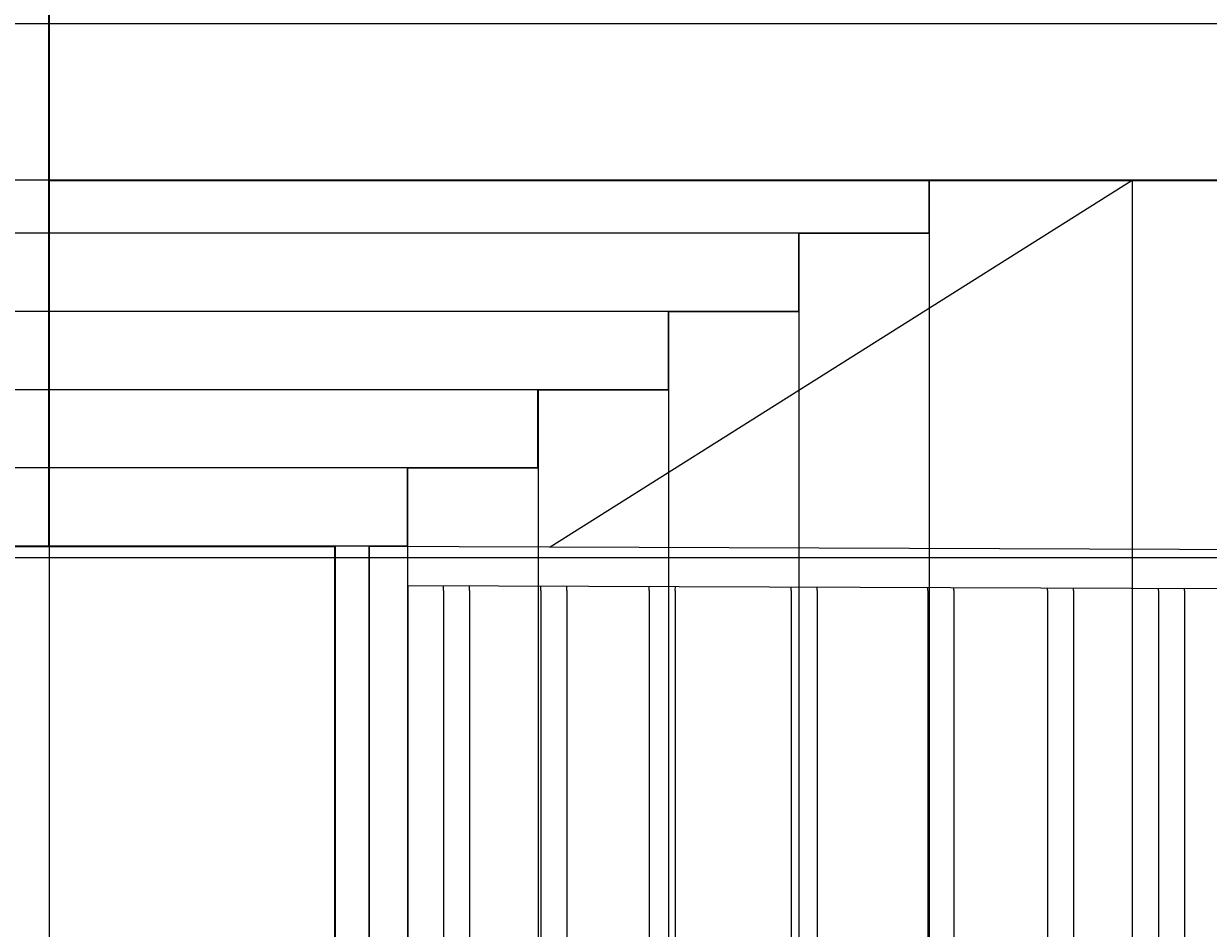
# Model space of a CAD drawing. Units: inches. Extents: x -13 to 809, y 112 to 656.
# Tile 19 of 55: x 339 to 430, y 181 to 251. Entities that reach past the tile are written whole.
import ezdxf

# ---------------------------------------------------------------- set-up
doc = ezdxf.new("R2010")
doc.units = ezdxf.units.IN
doc.header["$MEASUREMENT"] = 0
for name, color, linetype, lineweight in [('A-ANNO-DIMS', 2, 'Continuous', 18), ('A-DOOR', 4, 'Continuous', 25), ('A-ELEV', 7, 'Continuous', 35), ('A-FLOR-STRS', 3, 'Continuous', 25)]:
    doc.layers.add(name, color=color, linetype=linetype, lineweight=lineweight)
doc.styles.get("Standard").update_dxf_attribs({"font": 'arial.ttf'})
doc.dimstyles.get("Standard").update_dxf_attribs({"dimtxt": 0.625, "dimasz": 0.18, "dimexe": 0.18, "dimexo": 0.0625, "dimgap": 0.09, "dimtad": 0, "dimtih": 1, "dimtoh": 1, "dimdec": 4, "dimzin": 0, "dimdsep": 46, "dimlunit": 4, "dimtxsty": 'Standard', "dimcen": 0.09, "dimadec": 0, "dimazin": 0, "dimtfac": 1, "dimtdec": 4, "dimtofl": 0, "dimtmove": 0, "dimatfit": 3, "dimfxl": 1, "dimtolj": 1, "dimtzin": 0, "dimarcsym": 0})

# ---------------------------------------------------------------- blocks, each defined once
blk = doc.blocks.new('*D19')
at = {"layer": 'A-ANNO-DIMS', "color": 0, "lineweight": -2, "transparency": 16777216}
for p, q in [((337.507, 306.457), (337.507, 112.34)), ((365.938, 210.722), (365.938, 112.34)), ((337.687, 112.52), (350.573, 112.52)), ((365.758, 112.52), (352.873, 112.52))]:
    blk.add_line(p, q, dxfattribs=at)
at = {"layer": 'A-ANNO-DIMS', "color": 0, "transparency": 16777216}
for points in [[(337.687, 112.55), (337.687, 112.49), (337.507, 112.52)], [(365.758, 112.55), (365.758, 112.49), (365.938, 112.52)]]:
    blk.add_solid(points, dxfattribs=at)
at = {"layer": 'Defpoints', "color": 0, "transparency": 16777216}
for p in [(337.507, 306.52), (365.938, 210.785), (365.938, 112.52)]:
    blk.add_point(p, dxfattribs=at)
at = {"layer": 'A-ANNO-DIMS', "color": 0, "transparency": 16777216, "insert": (351.723, 112.52), "char_height": 0.625, "attachment_point": 5}
blk.add_mtext('\\A1;28.43', dxfattribs=at)
blk = doc.blocks.new('*D20')
at = {"layer": 'A-ANNO-DIMS', "color": 0, "lineweight": -2, "transparency": 16777216}
for p, q in [((365.938, 210.722), (365.938, 112.34)), ((607.574, 209.813), (607.574, 112.34)), ((366.118, 112.52), (485.365, 112.52)), ((607.394, 112.52), (488.148, 112.52))]:
    blk.add_line(p, q, dxfattribs=at)
at = {"layer": 'A-ANNO-DIMS', "color": 0, "transparency": 16777216}
for points in [[(366.118, 112.55), (366.118, 112.49), (365.938, 112.52)], [(607.394, 112.55), (607.394, 112.49), (607.574, 112.52)]]:
    blk.add_solid(points, dxfattribs=at)
at = {"layer": 'Defpoints', "color": 0, "transparency": 16777216}
for p in [(365.938, 210.785), (607.574, 209.875), (607.574, 112.52)]:
    blk.add_point(p, dxfattribs=at)
at = {"layer": 'A-ANNO-DIMS', "color": 0, "transparency": 16777216, "insert": (486.756, 112.52), "char_height": 0.625, "attachment_point": 5}
blk.add_mtext('\\A1;241.64', dxfattribs=at)
blk = doc.blocks.new('*D49')
at = {"layer": 'A-ANNO-DIMS', "color": 0, "lineweight": -2, "transparency": 16777216}
for p, q in [((590.946, 250.843), (-12.099, 250.843)), ((-11.919, 250.663), (-11.919, 245.247)), ((-11.919, 239.023), (-11.919, 244.439)), ((590.946, 238.843), (-12.099, 238.843))]:
    blk.add_line(p, q, dxfattribs=at)
at = {"layer": 'A-ANNO-DIMS', "color": 0, "transparency": 16777216}
for points in [[(-11.949, 250.663), (-11.889, 250.663), (-11.919, 250.843)], [(-11.949, 239.023), (-11.889, 239.023), (-11.919, 238.843)]]:
    blk.add_solid(points, dxfattribs=at)
at = {"layer": 'Defpoints', "color": 0, "transparency": 16777216}
for p in [(-11.919, 250.843), (591.008, 250.843), (591.008, 238.843)]:
    blk.add_point(p, dxfattribs=at)
at = {"layer": 'A-ANNO-DIMS', "color": 0, "transparency": 16777216, "insert": (-11.919, 244.843), "char_height": 0.625, "attachment_point": 5}
blk.add_mtext('\\A1;12', dxfattribs=at)
blk = doc.blocks.new('*D50')
at = {"layer": 'A-ANNO-DIMS', "color": 0, "lineweight": -2, "transparency": 16777216}
for p, q in [((590.946, 238.843), (-12.099, 238.843)), ((-11.919, 238.663), (-11.919, 224.768)), ((-11.919, 210.055), (-11.919, 223.95)), ((607.512, 209.875), (-12.099, 209.875))]:
    blk.add_line(p, q, dxfattribs=at)
at = {"layer": 'A-ANNO-DIMS', "color": 0, "transparency": 16777216}
for points in [[(-11.949, 238.663), (-11.889, 238.663), (-11.919, 238.843)], [(-11.949, 210.055), (-11.889, 210.055), (-11.919, 209.875)]]:
    blk.add_solid(points, dxfattribs=at)
at = {"layer": 'Defpoints', "color": 0, "transparency": 16777216}
for p in [(591.008, 238.843), (-11.919, 209.875), (607.574, 209.875)]:
    blk.add_point(p, dxfattribs=at)
at = {"layer": 'A-ANNO-DIMS', "color": 0, "transparency": 16777216, "insert": (-11.919, 224.359), "char_height": 0.625, "attachment_point": 5}
blk.add_mtext('\\A1;28.97', dxfattribs=at)
blk = doc.blocks.new('*D51')
at = {"layer": 'A-ANNO-DIMS', "color": 0, "lineweight": -2, "transparency": 16777216}
for p, q in [((341.407, 288.388), (341.407, 112.34)), ((442.184, 288.388), (442.184, 112.34)), ((341.587, 112.52), (390.437, 112.52)), ((442.004, 112.52), (393.154, 112.52))]:
    blk.add_line(p, q, dxfattribs=at)
at = {"layer": 'A-ANNO-DIMS', "color": 0, "transparency": 16777216}
for points in [[(341.587, 112.55), (341.587, 112.49), (341.407, 112.52)], [(442.004, 112.55), (442.004, 112.49), (442.184, 112.52)]]:
    blk.add_solid(points, dxfattribs=at)
at = {"layer": 'Defpoints', "color": 0, "transparency": 16777216}
for p in [(341.407, 288.451), (442.184, 288.451), (442.184, 112.52)]:
    blk.add_point(p, dxfattribs=at)
at = {"layer": 'A-ANNO-DIMS', "color": 0, "transparency": 16777216, "insert": (391.796, 112.52), "char_height": 0.625, "attachment_point": 5}
blk.add_mtext('\\A1;100.78', dxfattribs=at)
blk = doc.blocks.new('*D74')
at = {"layer": 'A-ANNO-DIMS', "color": 0, "lineweight": -2, "transparency": 16777216}
for p, q in [((341.407, 210.722), (341.407, 112.34)), ((368.897, 210.711), (368.897, 112.34)), ((341.587, 112.52), (354.001, 112.52)), ((368.717, 112.52), (356.302, 112.52))]:
    blk.add_line(p, q, dxfattribs=at)
at = {"layer": 'A-ANNO-DIMS', "color": 0, "transparency": 16777216}
for points in [[(341.587, 112.55), (341.587, 112.49), (341.407, 112.52)], [(368.717, 112.55), (368.717, 112.49), (368.897, 112.52)]]:
    blk.add_solid(points, dxfattribs=at)
at = {"layer": 'Defpoints', "color": 0, "transparency": 16777216}
for p in [(341.407, 210.785), (368.897, 210.774), (368.897, 112.52)]:
    blk.add_point(p, dxfattribs=at)
at = {"layer": 'A-ANNO-DIMS', "color": 0, "transparency": 16777216, "insert": (355.152, 112.52), "char_height": 0.625, "attachment_point": 5}
blk.add_mtext('\\A1;27.49', dxfattribs=at)
blk = doc.blocks.new('*D75')
at = {"layer": 'A-ANNO-DIMS', "color": 0, "lineweight": -2, "transparency": 16777216}
for p, q in [((378.897, 222.711), (378.897, 112.34)), ((368.897, 216.711), (368.897, 112.34)), ((369.077, 112.52), (373.389, 112.52)), ((378.717, 112.52), (374.404, 112.52))]:
    blk.add_line(p, q, dxfattribs=at)
at = {"layer": 'A-ANNO-DIMS', "color": 0, "transparency": 16777216}
for points in [[(369.077, 112.55), (369.077, 112.49), (368.897, 112.52)], [(378.717, 112.55), (378.717, 112.49), (378.897, 112.52)]]:
    blk.add_solid(points, dxfattribs=at)
at = {"layer": 'Defpoints', "color": 0, "transparency": 16777216}
for p in [(378.897, 222.774), (368.897, 216.774), (378.897, 112.52)]:
    blk.add_point(p, dxfattribs=at)
at = {"layer": 'A-ANNO-DIMS', "color": 0, "transparency": 16777216, "insert": (373.897, 112.52), "char_height": 0.625, "attachment_point": 5}
blk.add_mtext('\\A1;10', dxfattribs=at)
blk = doc.blocks.new('*D76')
at = {"layer": 'A-ANNO-DIMS', "color": 0, "lineweight": -2, "transparency": 16777216}
for p, q in [((388.897, 228.711), (388.897, 112.34)), ((378.897, 222.711), (378.897, 112.34)), ((379.077, 112.52), (383.389, 112.52)), ((388.717, 112.52), (384.404, 112.52))]:
    blk.add_line(p, q, dxfattribs=at)
at = {"layer": 'A-ANNO-DIMS', "color": 0, "transparency": 16777216}
for points in [[(379.077, 112.55), (379.077, 112.49), (378.897, 112.52)], [(388.717, 112.55), (388.717, 112.49), (388.897, 112.52)]]:
    blk.add_solid(points, dxfattribs=at)
at = {"layer": 'Defpoints', "color": 0, "transparency": 16777216}
for p in [(388.897, 228.774), (378.897, 222.774), (388.897, 112.52)]:
    blk.add_point(p, dxfattribs=at)
at = {"layer": 'A-ANNO-DIMS', "color": 0, "transparency": 16777216, "insert": (383.897, 112.52), "char_height": 0.625, "attachment_point": 5}
blk.add_mtext('\\A1;10', dxfattribs=at)
blk = doc.blocks.new('*D77')
at = {"layer": 'A-ANNO-DIMS', "color": 0, "lineweight": -2, "transparency": 16777216}
for p, q in [((398.897, 234.711), (398.897, 112.34)), ((388.897, 228.711), (388.897, 112.34)), ((389.077, 112.52), (393.389, 112.52)), ((398.717, 112.52), (394.404, 112.52))]:
    blk.add_line(p, q, dxfattribs=at)
at = {"layer": 'A-ANNO-DIMS', "color": 0, "transparency": 16777216}
for points in [[(389.077, 112.55), (389.077, 112.49), (388.897, 112.52)], [(398.717, 112.55), (398.717, 112.49), (398.897, 112.52)]]:
    blk.add_solid(points, dxfattribs=at)
at = {"layer": 'Defpoints', "color": 0, "transparency": 16777216}
for p in [(398.897, 234.774), (388.897, 228.774), (398.897, 112.52)]:
    blk.add_point(p, dxfattribs=at)
at = {"layer": 'A-ANNO-DIMS', "color": 0, "transparency": 16777216, "insert": (393.897, 112.52), "char_height": 0.625, "attachment_point": 5}
blk.add_mtext('\\A1;10', dxfattribs=at)
blk = doc.blocks.new('*D78')
at = {"layer": 'A-ANNO-DIMS', "color": 0, "lineweight": -2, "transparency": 16777216}
for p, q in [((408.897, 238.78), (408.897, 112.34)), ((398.897, 234.711), (398.897, 112.34)), ((399.077, 112.52), (403.389, 112.52)), ((408.717, 112.52), (404.404, 112.52))]:
    blk.add_line(p, q, dxfattribs=at)
at = {"layer": 'A-ANNO-DIMS', "color": 0, "transparency": 16777216}
for points in [[(399.077, 112.55), (399.077, 112.49), (398.897, 112.52)], [(408.717, 112.55), (408.717, 112.49), (408.897, 112.52)]]:
    blk.add_solid(points, dxfattribs=at)
at = {"layer": 'Defpoints', "color": 0, "transparency": 16777216}
for p in [(408.897, 238.843), (398.897, 234.774), (408.897, 112.52)]:
    blk.add_point(p, dxfattribs=at)
at = {"layer": 'A-ANNO-DIMS', "color": 0, "transparency": 16777216, "insert": (403.897, 112.52), "char_height": 0.625, "attachment_point": 5}
blk.add_mtext('\\A1;10', dxfattribs=at)
blk = doc.blocks.new('*D79')
at = {"layer": 'A-ANNO-DIMS', "color": 0, "lineweight": -2, "transparency": 16777216}
for p, q in [((408.897, 238.78), (408.897, 112.34)), ((424.469, 238.78), (424.469, 112.34)), ((409.077, 112.52), (415.328, 112.52)), ((424.289, 112.52), (418.037, 112.52))]:
    blk.add_line(p, q, dxfattribs=at)
at = {"layer": 'A-ANNO-DIMS', "color": 0, "transparency": 16777216}
for points in [[(409.077, 112.55), (409.077, 112.49), (408.897, 112.52)], [(424.289, 112.55), (424.289, 112.49), (424.469, 112.52)]]:
    blk.add_solid(points, dxfattribs=at)
at = {"layer": 'Defpoints', "color": 0, "transparency": 16777216}
for p in [(408.897, 238.843), (424.469, 238.843), (424.469, 112.52)]:
    blk.add_point(p, dxfattribs=at)
at = {"layer": 'A-ANNO-DIMS', "color": 0, "transparency": 16777216, "insert": (416.683, 112.52), "char_height": 0.625, "attachment_point": 5}
blk.add_mtext('\\A1;15.572', dxfattribs=at)
blk = doc.blocks.new('*D80')
at = {"layer": 'A-ANNO-DIMS', "color": 0, "lineweight": -2, "transparency": 16777216}
for p, q in [((368.834, 216.774), (-12.099, 216.774)), ((-11.919, 216.594), (-11.919, 214.183)), ((-11.919, 210.954), (-11.919, 213.365)), ((368.834, 210.774), (-12.099, 210.774))]:
    blk.add_line(p, q, dxfattribs=at)
at = {"layer": 'A-ANNO-DIMS', "color": 0, "transparency": 16777216}
for points in [[(-11.949, 216.594), (-11.889, 216.594), (-11.919, 216.774)], [(-11.949, 210.954), (-11.889, 210.954), (-11.919, 210.774)]]:
    blk.add_solid(points, dxfattribs=at)
at = {"layer": 'Defpoints', "color": 0, "transparency": 16777216}
for p in [(-11.919, 216.774), (368.897, 216.774), (368.897, 210.774)]:
    blk.add_point(p, dxfattribs=at)
at = {"layer": 'A-ANNO-DIMS', "color": 0, "transparency": 16777216, "insert": (-11.919, 213.774), "char_height": 0.625, "attachment_point": 5}
blk.add_mtext('\\A1;6', dxfattribs=at)
blk = doc.blocks.new('*D81')
at = {"layer": 'A-ANNO-DIMS', "color": 0, "lineweight": -2, "transparency": 16777216}
for p, q in [((378.834, 222.774), (-12.099, 222.774)), ((-11.919, 222.594), (-11.919, 220.183)), ((-11.919, 216.954), (-11.919, 219.365)), ((378.834, 216.774), (-12.099, 216.774))]:
    blk.add_line(p, q, dxfattribs=at)
at = {"layer": 'A-ANNO-DIMS', "color": 0, "transparency": 16777216}
for points in [[(-11.949, 222.594), (-11.889, 222.594), (-11.919, 222.774)], [(-11.949, 216.954), (-11.889, 216.954), (-11.919, 216.774)]]:
    blk.add_solid(points, dxfattribs=at)
at = {"layer": 'Defpoints', "color": 0, "transparency": 16777216}
for p in [(-11.919, 222.774), (378.897, 222.774), (378.897, 216.774)]:
    blk.add_point(p, dxfattribs=at)
at = {"layer": 'A-ANNO-DIMS', "color": 0, "transparency": 16777216, "insert": (-11.919, 219.774), "char_height": 0.625, "attachment_point": 5}
blk.add_mtext('\\A1;6', dxfattribs=at)
blk = doc.blocks.new('*D82')
at = {"layer": 'A-ANNO-DIMS', "color": 0, "lineweight": -2, "transparency": 16777216}
for p, q in [((388.834, 228.774), (-12.099, 228.774)), ((-11.919, 228.594), (-11.919, 226.183)), ((-11.919, 222.954), (-11.919, 225.365)), ((388.834, 222.774), (-12.099, 222.774))]:
    blk.add_line(p, q, dxfattribs=at)
at = {"layer": 'A-ANNO-DIMS', "color": 0, "transparency": 16777216}
for points in [[(-11.949, 228.594), (-11.889, 228.594), (-11.919, 228.774)], [(-11.949, 222.954), (-11.889, 222.954), (-11.919, 222.774)]]:
    blk.add_solid(points, dxfattribs=at)
at = {"layer": 'Defpoints', "color": 0, "transparency": 16777216}
for p in [(-11.919, 228.774), (388.897, 228.774), (388.897, 222.774)]:
    blk.add_point(p, dxfattribs=at)
at = {"layer": 'A-ANNO-DIMS', "color": 0, "transparency": 16777216, "insert": (-11.919, 225.774), "char_height": 0.625, "attachment_point": 5}
blk.add_mtext('\\A1;6', dxfattribs=at)
blk = doc.blocks.new('*D83')
at = {"layer": 'A-ANNO-DIMS', "color": 0, "lineweight": -2, "transparency": 16777216}
for p, q in [((398.834, 234.774), (-12.099, 234.774)), ((-11.919, 234.594), (-11.919, 232.183)), ((-11.919, 228.954), (-11.919, 231.365)), ((398.834, 228.774), (-12.099, 228.774))]:
    blk.add_line(p, q, dxfattribs=at)
at = {"layer": 'A-ANNO-DIMS', "color": 0, "transparency": 16777216}
for points in [[(-11.949, 234.594), (-11.889, 234.594), (-11.919, 234.774)], [(-11.949, 228.954), (-11.889, 228.954), (-11.919, 228.774)]]:
    blk.add_solid(points, dxfattribs=at)
at = {"layer": 'Defpoints', "color": 0, "transparency": 16777216}
for p in [(-11.919, 234.774), (398.897, 234.774), (398.897, 228.774)]:
    blk.add_point(p, dxfattribs=at)
at = {"layer": 'A-ANNO-DIMS', "color": 0, "transparency": 16777216, "insert": (-11.919, 231.774), "char_height": 0.625, "attachment_point": 5}
blk.add_mtext('\\A1;6', dxfattribs=at)
blk = doc.blocks.new('*D84')
at = {"layer": 'A-ANNO-DIMS', "color": 0, "lineweight": -2, "transparency": 16777216}
for p, q in [((408.834, 238.843), (-12.099, 238.843)), ((-11.919, 238.663), (-11.919, 237.217)), ((-11.919, 234.954), (-11.919, 236.399)), ((408.834, 234.774), (-12.099, 234.774))]:
    blk.add_line(p, q, dxfattribs=at)
at = {"layer": 'A-ANNO-DIMS', "color": 0, "transparency": 16777216}
for points in [[(-11.949, 238.663), (-11.889, 238.663), (-11.919, 238.843)], [(-11.949, 234.954), (-11.889, 234.954), (-11.919, 234.774)]]:
    blk.add_solid(points, dxfattribs=at)
at = {"layer": 'Defpoints', "color": 0, "transparency": 16777216}
for p in [(-11.919, 238.843), (408.897, 238.843), (408.897, 234.774)]:
    blk.add_point(p, dxfattribs=at)
at = {"layer": 'A-ANNO-DIMS', "color": 0, "transparency": 16777216, "insert": (-11.919, 236.808), "char_height": 0.625, "attachment_point": 5}
blk.add_mtext('\\A1;4.069', dxfattribs=at)

msp = doc.modelspace()

# ---------------------------------------------------------------- linework, layer by layer
at = {"layer": 'A-DOOR'}
for p, q in [((371.6498, 207.3724), (371.6513, 207.7634)), ((371.6498, 207.3724), (371.6498, 155.2141)), ((373.6498, 207.3724), (373.6513, 207.7559)), ((373.6498, 207.3724), (373.6498, 155.2141)), ((379.1123, 207.3724), (379.1136, 207.7353)), ((379.1123, 207.3724), (379.1123, 155.2141)), ((381.1123, 207.3724), (381.1136, 207.7278)), ((381.1123, 207.3724), (381.1123, 155.2141)), ((387.4276, 207.3724), (387.4288, 207.704)), ((387.4276, 207.3724), (387.4276, 155.2141)), ((389.4276, 207.3724), (389.4288, 207.6965)), ((389.4276, 207.3724), (389.4276, 155.2141)), ((398.3015, 207.3724), (398.3026, 207.6631)), ((398.3015, 207.3724), (398.3015, 155.2141)), ((400.3015, 207.3724), (400.3025, 207.6556)), ((400.3015, 207.3724), (400.3015, 155.2141)), ((408.7873, 207.3724), (408.7882, 207.6236)), ((408.7873, 207.3724), (408.7873, 155.2141)), ((410.7873, 207.3724), (410.7882, 207.6161)), ((410.7873, 207.3724), (410.7873, 155.2141)), ((417.9555, 207.3724), (417.9563, 207.5891)), ((417.9555, 207.3724), (417.9555, 155.2141)), ((419.9555, 207.3724), (419.9563, 207.5816)), ((419.9555, 207.3724), (419.9555, 155.2141)), ((426.484, 207.3724), (426.4847, 207.557)), ((426.484, 207.3724), (426.484, 155.2141)), ((428.484, 207.3724), (428.4847, 207.5495)), ((428.484, 207.3724), (428.484, 155.2141))]:
    msp.add_line(p, q, dxfattribs=at)
for points in [[(365.9383, 210.7849), (607.5741, 209.8753), (607.5741, 152.2141), (365.9383, 152.2141)], [(368.9383, 207.7736), (604.5741, 206.8866), (604.5741, 155.2141), (368.9383, 155.2141)]]:
    msp.add_lwpolyline(points, close=True, dxfattribs=at)
at = {"layer": 'A-ELEV'}
for p, q in [((341.4072, 210.7849), (341.4072, 524.281)), ((341.4072, 238.8429), (591.008, 238.8429)), ((311.6991, 210.7849), (363.3158, 210.7849)), ((363.3158, 210.7849), (363.3158, 150.5199))]:
    msp.add_line(p, q, dxfattribs=at)
at = {"layer": 'A-FLOR-STRS'}
for p, q in [((379.8204, 210.7327), (424.469, 238.8429)), ((408.8966, 234.7738), (408.8966, 238.8429)), ((398.8966, 228.7738), (398.8966, 234.7738)), ((398.8966, 234.7738), (408.8966, 234.7738)), ((388.8966, 222.7738), (388.8966, 228.7738)), ((388.8966, 228.7738), (398.8966, 228.7738)), ((378.8966, 216.7738), (378.8966, 222.7738)), ((378.8966, 222.7738), (388.8966, 222.7738)), ((368.8966, 210.7738), (368.8966, 216.7738)), ((368.8966, 216.7738), (378.8966, 216.7738))]:
    msp.add_line(p, q, dxfattribs=at)

# ---------------------------------------------------------------- dimensions: what is measured, and where the dimension line sits
at = {"layer": 'A-ANNO-DIMS'}
for base, p1, p2, override, picture, middle in [((365.9383, 112.5199), (337.5074, 306.5199), (365.9383, 210.7849), {"dimdec": 2, "dimlfac": 1, "dimrnd": 0, "dimzin": 0, "dimdsep": 46, "dimlunit": 2}, '*D19', (351.7228, 112.5199)), ((442.1845, 112.5199), (341.4072, 288.4508), (442.1845, 288.4508), {"dimdec": 2, "dimlfac": 1, "dimrnd": 0, "dimzin": 0, "dimdsep": 46, "dimlunit": 2}, '*D51', (391.7958, 112.5199)), ((408.8966, 112.5199), (398.8966, 234.7738), (408.8966, 238.8429), {"dimdec": 0, "dimlfac": 1, "dimrnd": 0, "dimzin": 0, "dimdsep": 46, "dimlunit": 2}, '*D78', (403.8966, 112.5199)), ((424.469, 112.5199), (408.8966, 238.8429), (424.469, 238.8429), {"dimdec": 3, "dimlfac": 1, "dimrnd": 0, "dimzin": 0, "dimdsep": 46, "dimlunit": 2}, '*D79', (416.6828, 112.5199)), ((398.8966, 112.5199), (388.8966, 228.7738), (398.8966, 234.7738), {"dimdec": 0, "dimlfac": 1, "dimrnd": 0, "dimzin": 0, "dimdsep": 46, "dimlunit": 2}, '*D77', (393.8966, 112.5199)), ((388.8966, 112.5199), (378.8966, 222.7738), (388.8966, 228.7738), {"dimdec": 0, "dimlfac": 1, "dimrnd": 0, "dimzin": 0, "dimdsep": 46, "dimlunit": 2}, '*D76', (383.8966, 112.5199)), ((378.8966, 112.5199), (368.8966, 216.7738), (378.8966, 222.7738), {"dimdec": 0, "dimlfac": 1, "dimrnd": 0, "dimzin": 0, "dimdsep": 46, "dimlunit": 2}, '*D75', (373.8966, 112.5199)), ((368.8966, 112.5199), (341.4072, 210.7849), (368.8966, 210.7738), {"dimdec": 2, "dimlfac": 1, "dimrnd": 0, "dimzin": 0, "dimdsep": 46, "dimlunit": 2}, '*D74', (355.1519, 112.5199)), ((607.5741, 112.5199), (365.9383, 210.7849), (607.5741, 209.8753), {"dimdec": 2, "dimlfac": 1, "dimrnd": 0, "dimzin": 0, "dimdsep": 46, "dimlunit": 2}, '*D20', (486.7562, 112.5199))]:
    dim = msp.add_linear_dim(base=base, p1=p1, p2=p2, dimstyle='Standard', override=override, dxfattribs=at)
    dim.commit()
    dim.dimension.update_dxf_attribs({"geometry": picture, "text_midpoint": middle})
for base, p1, p2, override, picture, middle in [((-11.9191, 250.8429), (591.008, 238.8429), (591.008, 250.8429), {"dimdec": 0, "dimlfac": 1, "dimrnd": 0, "dimzin": 0, "dimdsep": 46, "dimlunit": 2}, '*D49', (-11.9191, 244.8429)), ((-11.9191, 209.8753), (591.008, 238.8429), (607.5741, 209.8753), {"dimdec": 2, "dimlfac": 1, "dimrnd": 0, "dimzin": 0, "dimdsep": 46, "dimlunit": 2}, '*D50', (-11.9191, 224.3591)), ((-11.9191, 238.8429), (408.8966, 234.7738), (408.8966, 238.8429), {"dimdec": 3, "dimlfac": 1, "dimrnd": 0, "dimzin": 0, "dimdsep": 46, "dimlunit": 2}, '*D84', (-11.9191, 236.8083)), ((-11.9191, 234.7738), (398.8966, 228.7738), (398.8966, 234.7738), {"dimdec": 0, "dimlfac": 1, "dimrnd": 0, "dimzin": 0, "dimdsep": 46, "dimlunit": 2}, '*D83', (-11.9191, 231.7738)), ((-11.9191, 228.7738), (388.8966, 222.7738), (388.8966, 228.7738), {"dimdec": 0, "dimlfac": 1, "dimrnd": 0, "dimzin": 0, "dimdsep": 46, "dimlunit": 2}, '*D82', (-11.9191, 225.7738)), ((-11.9191, 222.7738), (378.8966, 216.7738), (378.8966, 222.7738), {"dimdec": 0, "dimlfac": 1, "dimrnd": 0, "dimzin": 0, "dimdsep": 46, "dimlunit": 2}, '*D81', (-11.9191, 219.7738)), ((-11.9191, 216.7738), (368.8966, 210.7738), (368.8966, 216.7738), {"dimdec": 0, "dimlfac": 1, "dimrnd": 0, "dimzin": 0, "dimdsep": 46, "dimlunit": 2}, '*D80', (-11.9191, 213.7738))]:
    dim = msp.add_linear_dim(base=base, p1=p1, p2=p2, angle=90, dimstyle='Standard', override=override, dxfattribs=at)
    dim.commit()
    dim.dimension.update_dxf_attribs({"geometry": picture, "text_midpoint": middle})

doc.saveas('drawing.dxf')
